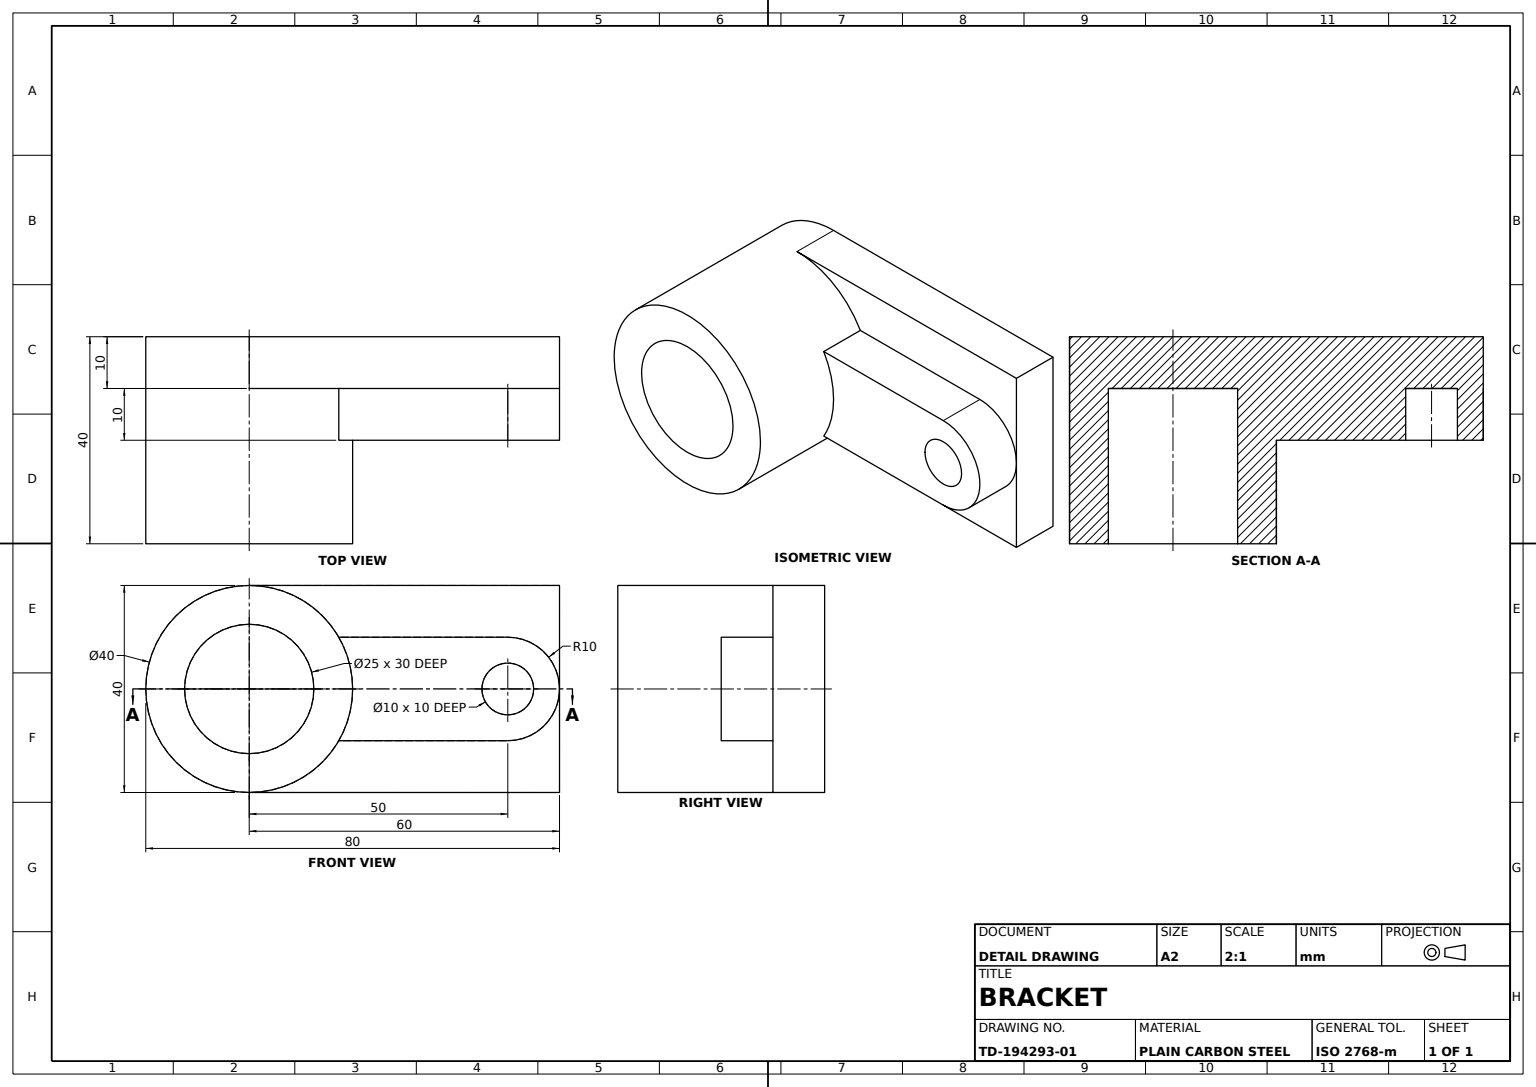
SolidWorks part; units mm, degrees
material "Plain Carbon Steel"
ref_plane "Front Plane" through (0, 0, 0) normal (0, 0, 1) x (1, 0, 0)
ref_plane "Top Plane" through (0, 0, 0) normal (0, 1, 0) x (1, 0, 0)
ref_plane "Right Plane" through (0, 0, 0) normal (1, 0, 0) x (0, 0, -1)
sketch "Base Plate Sketch" plane through (0, 0, 0) normal (0, 0, 1) x (1, 0, 0)
  line L0 (0, 0) -> (60, 0)
  line L1 (60, 0) -> (60, -40)
  line L2 (60, -40) -> (0, -40)
  line L3 (0, -40) -> (0, 0)
  dimension "D1" = 60
  dimension "D2" = 40
extrude "Base Plate" add sketch "Base Plate Sketch" along normal blind 10
sketch "Cylinder Boss Sketch Ø40" plane through (0, 0, 10) normal (0, 0, 1) x (1, 0, 0)
  line L0 (0, 0) -> (0, -40) construction
  circle A0 centre (0, -20) radius 20
  dimension "D1" = 40
  dimension "D2" = 40
extrude "Cylinder Boss Ø40" add sketch "Cylinder Boss Sketch Ø40" along normal blind 40
sketch "Cylinder Root Boss Sketch Ø40" plane through (0, 0, 0) normal (0, 0, -1) x (-1, 0, 0)
  line L0 (0, 0) -> (0, -40) construction
  circle A0 centre (0, -20) radius 20
  dimension "D1" = 40
  dimension "D2" = 40
extrude "Cylinder Root Boss Ø40" add sketch "Cylinder Root Boss Sketch Ø40" against normal blind 10
sketch "Cylinder Clearance Cut Sketch Ø40" plane through (0, 0, 50) normal (0, 0, 1) x (1, 0, 0)
  circle A0 centre (0, -20) radius 20
  dimension "D1" = 40
  dimension "D2" = 40
extrude "Cylinder Clearance Cut Ø40" cut sketch "Cylinder Clearance Cut Sketch Ø40" against normal blind 10
sketch "Lug Arm Sketch" plane through (0, 0, 10) normal (0, 0, 1) x (1, 0, 0)
  line L2 (50, -10) -> (17.3205, -10)
  line L3 (50, -30) -> (17.3205, -30)
  arc A0 (50, -30) -> (50, -10) centre (50, -20) ccw
  arc A1 (0, -40) -> (0, 0) centre (0, -20) ccw construction
  circle A2 centre (0, -20) radius 20 construction
  arc A3 (17.3205, -30) -> (17.3205, -10) centre (0, -20) ccw
  dimension "D1" = 20
  dimension "D2" = 40
  dimension "D3" = 10
  dimension "D4" = 50
extrude "Lug Arm" add sketch "Lug Arm Sketch" along normal blind 10
sketch "Lug Hole Sketch Ø10" plane through (0, 0, 20) normal (0, 0, 1) x (1, 0, 0)
  circle A0 centre (50, -20) radius 5
  dimension "D1" = 10
  dimension "D2" = 10
extrude "Lug Hole Ø10" cut sketch "Lug Hole Sketch Ø10" against normal blind 10
sketch "Bore Sketch Ø25" plane through (0, 0, 40) normal (0, 0, 1) x (1, 0, 0)
  circle A0 centre (0, -20) radius 12.5
  dimension "D1" = 25
  dimension "D2" = 25
extrude "Bore Ø25" cut sketch "Bore Sketch Ø25" against normal blind 30
